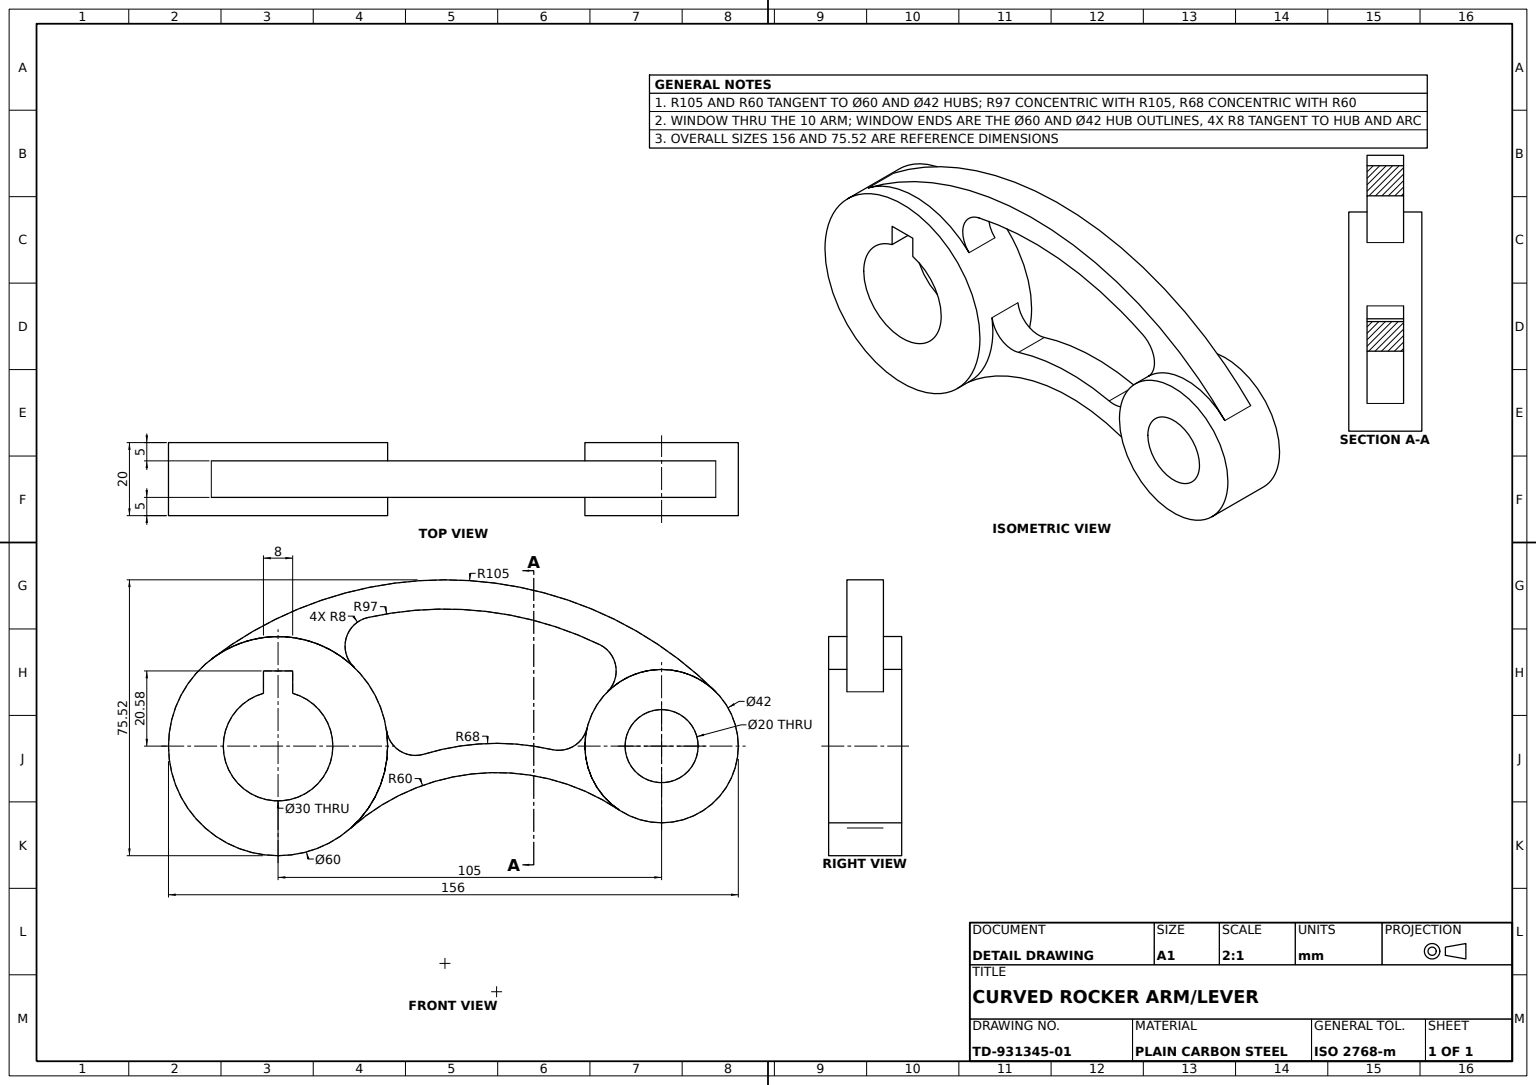
from build123d import *

# Parameters (mm, degrees)
HUB_BOSSES_20MM_DEPTH        = 10
HUB_BOSSES_20MM_DEPTH_BACK   = 10
HUB_BOSSES_20MM_2_DEPTH      = 10
HUB_BOSSES_20MM_2_DEPTH_BACK = 10
LEVER_PROFILE_SKETCH_R       = 10
ARM_WEB_10MM_DEPTH           = 5
ARM_WEB_10MM_DEPTH_BACK      = 5


with BuildPart() as part:
    # Lever Profile Sketch → Hub Bosses 20mm (new, two sides: drawn at the far end of the back side and taken through both)
    with BuildSketch(Plane.XY.offset(-HUB_BOSSES_20MM_DEPTH_BACK)):
        with BuildLine():
            ThreePointArc((-123.274285714, 23.791815434), (-128.116796704, -19.121027957), (-85.057142857, -22.411658773))
            ThreePointArc((-85.057142857, -22.411658773), (-77.629525814, -12.282391577), (-75, 0))
            ThreePointArc((-75, 0), (-75.077467799, 2.154545592), (-75.309471114, 4.297963991))
            ThreePointArc((-75.309471114, 4.297963991), (-78.312822706, 13.703815821), (-84.206993671, 21.625237289))
            ThreePointArc((-84.206993671, 21.625237289), (-103.338824634, 29.953972965), (-123.274285714, 23.791815434))
        make_face()
        with BuildLine():
            Line((-109, 14.456832295), (-109, 20.578458237))
            Line((-109, 20.578458237), (-101, 20.578458237))
            Line((-101, 20.578458237), (-101, 14.456832295))
            ThreePointArc((-101, 14.456832295), (-105, -15), (-109, 14.456832295))
        make_face(mode=Mode.SUBTRACT)
    extrude(amount=HUB_BOSSES_20MM_DEPTH + HUB_BOSSES_20MM_DEPTH_BACK)



with BuildPart() as body_2:
    # Lever Profile Sketch → Hub Bosses 20mm 2 (new, two sides: drawn at the far end of the back side and taken through both)
    with BuildSketch(Plane.XY.offset(-HUB_BOSSES_20MM_2_DEPTH_BACK)):
        with BuildLine():
            ThreePointArc((-20.407235595, 4.954264362), (-19.57486428, -7.604254627), (-11.711111111, -17.431290157))
            ThreePointArc((-11.711111111, -17.431290157), (9.875896584, -18.532853711), (21, 0))
            ThreePointArc((21, 0), (19.39587585, 8.049844719), (14.828571429, 14.869884646))
            ThreePointArc((14.828571429, 14.869884646), (0.022511477, 20.999987934), (-14.796657075, 14.901642172))
            ThreePointArc((-14.796657075, 14.901642172), (-18.291148026, 10.316680857), (-20.407235595, 4.954264362))
        make_face()
        Circle(LEVER_PROFILE_SKETCH_R, mode=Mode.SUBTRACT)
    extrude(amount=HUB_BOSSES_20MM_2_DEPTH + HUB_BOSSES_20MM_2_DEPTH_BACK)


with BuildPart() as part_1:
    add(part.part)

    add(body_2.part)  # Arm Web 10mm merges body 2
    # Sketch1_6 → Arm Web 10mm (add, two sides: drawn at the far end of the back side and taken through both)
    with BuildSketch(Plane.XY.offset(-ARM_WEB_10MM_DEPTH_BACK)):
        with BuildLine():
            ThreePointArc((-85.057142857, -22.411658773), (-49.236210113, -7.37282174), (-11.711111111, -17.431290157))
            ThreePointArc((-11.711111111, -17.431290157), (-19.57486428, -7.604254627), (-20.407235595, 4.954264362))
            ThreePointArc((-20.407235595, 4.954264362), (-23.975479097, 0.036453925), (-29.969842477, -0.955931516))
            ThreePointArc((-29.969842477, -0.955931516), (-47.593498278, 0.721874536), (-65.052989568, -2.206340072))
            ThreePointArc((-65.052989568, -2.206340072), (-71.676423998, -1.311923165), (-75.309471114, 4.297963991))
            ThreePointArc((-75.309471114, 4.297963991), (-75.077467799, 2.154545592), (-75, 0))
            ThreePointArc((-75, 0), (-77.629525814, -12.282391577), (-85.057142857, -22.411658773))
        make_face()
        with BuildLine():
            ThreePointArc((-14.796657075, 14.901642172), (0.022511477, 20.999987934), (14.828571429, 14.869884646))
            ThreePointArc((14.828571429, 14.869884646), (-52.545027473, 45.302030133), (-123.274285714, 23.791815434))
            ThreePointArc((-123.274285714, 23.791815434), (-103.338824634, 29.953972965), (-84.206993671, 21.625237289))
            ThreePointArc((-84.206993671, 21.625237289), (-86.365233313, 29.551401021), (-80.401329626, 35.200641913))
            ThreePointArc((-80.401329626, 35.200641913), (-48.040951998, 36.863141194), (-16.938574827, 27.77468267))
            ThreePointArc((-16.938574827, 27.77468267), (-12.541970936, 21.891509402), (-14.796657075, 14.901642172))
        make_face()
    extrude(amount=ARM_WEB_10MM_DEPTH + ARM_WEB_10MM_DEPTH_BACK)


solid = part_1.part
